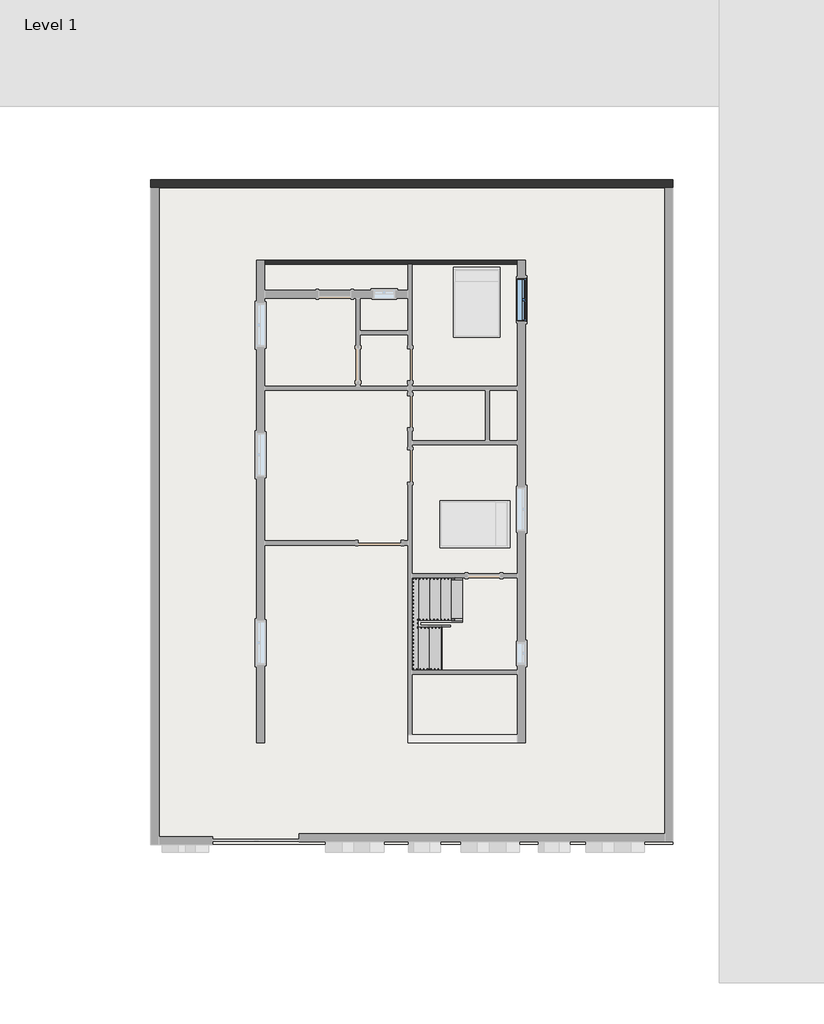
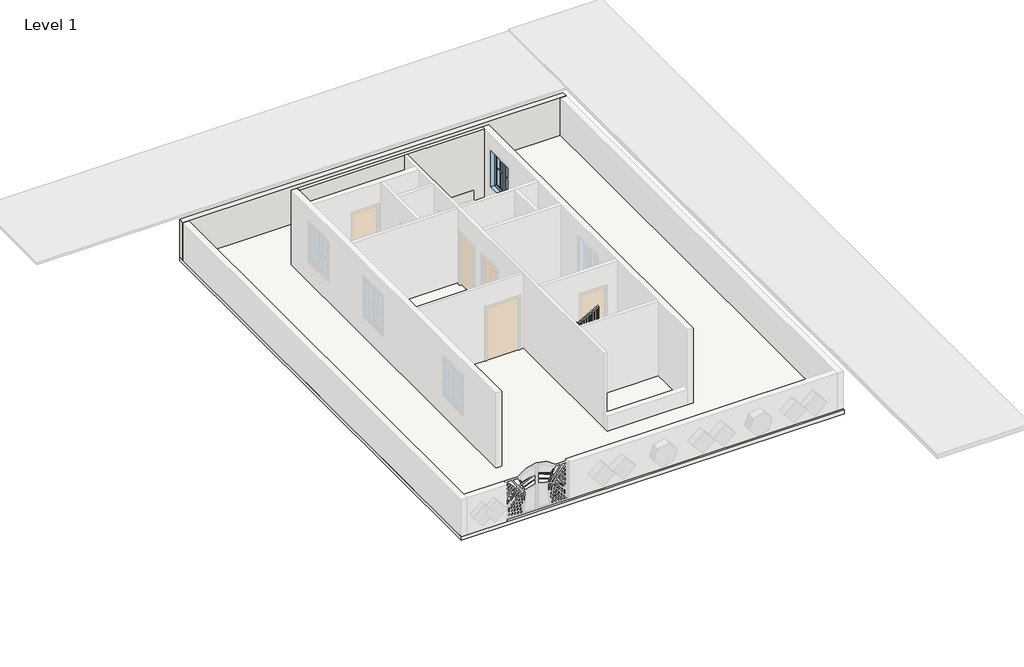
# One storey, part 2 of 7: 2 railings, 2 walls, 1 slab, 1 stair flight, 1 window.
"""IFC4 building model written with IfcOpenShell, lengths in millimetres."""

from ifc_helpers import new_model, si_unit, frame, origin, place, context, project, spatial, polyline, outline, extrude, faceted_brep, transform, mapped, element, save
from components import stair_flight_e4a46180, window_8377141f

model = new_model("IFC4")

# Units and contexts
model_context = context("Model", 3, world=origin())
ifc_project = project(units=[si_unit("LENGTHUNIT", "METRE", prefix="MILLI")], contexts=[model_context])

# Site, building, storey
site = spatial("IfcSite", under=ifc_project)
building = spatial("IfcBuilding", under=site)
storey = spatial("IfcBuildingStorey", under=building, Name="Level 1", Elevation=0.0)

# Railings
placement = place(None, origin())
element("IfcRailing", 1, ObjectType="Handrail - Rectangular", at=placement, inside=storey, context=model_context, shape_type="SolidModel", body=[
    faceted_brep([(7105.1820958, 5435.6, 1083.7333333), (7105.1820958, 5435.6, 1025.8977421), (7105.1820958, 5486.4, 1025.8977421), (7105.1820958, 5486.4, 1083.7333333), (5860.5820958, 5435.6, 1761.0666667), (5847.654197, 5435.6, 1710.2666667), (5847.654197, 5486.4, 1710.2666667), (5860.5820958, 5486.4, 1761.0666667), (5727.7, 5435.6, 1761.0666667), (5727.7, 5435.6, 1710.2666667), (5676.9, 5486.4, 1710.2666667), (5676.9, 5486.4, 1761.0666667), (5727.7, 2997.2, 1761.0666667), (5727.7, 2946.4, 1710.2666667), (5676.9, 2946.4, 1710.2666667), (5676.9, 2997.2, 1761.0666667), (5727.7, 2997.2, 1899.5526009), (5727.7, 2946.4, 1848.7526009), (5676.9, 2946.4, 1848.7526009), (5676.9, 2997.2, 1899.5526009), (5727.7, 2921.0, 1899.5526009), (5727.7, 2921.0, 1848.7526009), (5676.9, 2870.2, 1848.7526009), (5676.9, 2870.2, 1899.5526009), (5803.9, 2921.0, 1899.5526009), (5816.8278988, 2921.0, 1848.7526009), (5816.8278988, 2870.2, 1848.7526009), (5803.9, 2870.2, 1899.5526009), (7105.1820958, 2921.0, 2607.7333333), (7105.1820958, 2870.2, 2607.7333333), (7105.1820958, 2870.2, 2549.8977421), (7105.1820958, 2921.0, 2549.8977421)], [[[0, 1, 2, 3]], [[1, 0, 4, 5]], [[2, 1, 5, 6]], [[3, 2, 6, 7]], [[0, 3, 7, 4]], [[5, 4, 8, 9]], [[6, 5, 9, 10]], [[7, 6, 10, 11]], [[4, 7, 11, 8]], [[9, 8, 12, 13]], [[10, 9, 13, 14]], [[11, 10, 14, 15]], [[8, 11, 15, 12]], [[13, 12, 16, 17]], [[14, 13, 17, 18]], [[15, 14, 18, 19]], [[12, 15, 19, 16]], [[17, 16, 20, 21]], [[18, 17, 21, 22]], [[19, 18, 22, 23]], [[16, 19, 23, 20]], [[21, 20, 24, 25]], [[22, 21, 25, 26]], [[23, 22, 26, 27]], [[20, 23, 27, 24]], [[28, 29, 30, 31]], [[25, 24, 28, 31]], [[26, 25, 31, 30]], [[27, 26, 30, 29]], [[24, 27, 29, 28]]]),
    extrude(outline(polyline([(2510.4108873, 7032.625), (2500.0435403, 7013.575), (1524.0, 7013.575), (1524.0, 7032.625), (2510.4108873, 7032.625)])), frame((0.0, 2886.075, 0.0), z_axis=(0.0, 1.0, 0.0), x_axis=(0.0, 0.0, 1.0)), (0.0, 0.0, 1.0), 19.05),
    extrude(outline(polyline([(2455.1183703, 6931.025), (2444.7510233, 6911.975), (1524.0, 6911.975), (1524.0, 6931.025), (2455.1183703, 6931.025)])), frame((0.0, 2886.075, 0.0), z_axis=(0.0, 1.0, 0.0), x_axis=(0.0, 0.0, 1.0)), (0.0, 0.0, 1.0), 19.05),
    extrude(outline(polyline([(2399.8258533, 6829.425), (2389.4585063, 6810.375), (1524.0, 6810.375), (1524.0, 6829.425), (2399.8258533, 6829.425)])), frame((0.0, 2886.075, 0.0), z_axis=(0.0, 1.0, 0.0), x_axis=(0.0, 0.0, 1.0)), (0.0, 0.0, 1.0), 19.05),
    extrude(outline(polyline([(2344.5333363, 6727.825), (2334.1659893, 6708.775), (1354.6666667, 6708.775), (1354.6666667, 6727.825), (2344.5333363, 6727.825)])), frame((0.0, 2886.075, 0.0), z_axis=(0.0, 1.0, 0.0), x_axis=(0.0, 0.0, 1.0)), (0.0, 0.0, 1.0), 19.05),
    extrude(outline(polyline([(2289.2408192, 6626.225), (2278.8734723, 6607.175), (1354.6666667, 6607.175), (1354.6666667, 6626.225), (2289.2408192, 6626.225)])), frame((0.0, 2886.075, 0.0), z_axis=(0.0, 1.0, 0.0), x_axis=(0.0, 0.0, 1.0)), (0.0, 0.0, 1.0), 19.05),
    extrude(outline(polyline([(2233.9483022, 6524.625), (2223.5809553, 6505.575), (1354.6666667, 6505.575), (1354.6666667, 6524.625), (2233.9483022, 6524.625)])), frame((0.0, 2886.075, 0.0), z_axis=(0.0, 1.0, 0.0), x_axis=(0.0, 0.0, 1.0)), (0.0, 0.0, 1.0), 19.05),
    extrude(outline(polyline([(2178.6557852, 6423.025), (2168.2884383, 6403.975), (1185.3333333, 6403.975), (1185.3333333, 6423.025), (2178.6557852, 6423.025)])), frame((0.0, 2886.075, 0.0), z_axis=(0.0, 1.0, 0.0), x_axis=(0.0, 0.0, 1.0)), (0.0, 0.0, 1.0), 19.05),
    extrude(outline(polyline([(2123.3632682, 6321.425), (2112.9959213, 6302.375), (1185.3333333, 6302.375), (1185.3333333, 6321.425), (2123.3632682, 6321.425)])), frame((0.0, 2886.075, 0.0), z_axis=(0.0, 1.0, 0.0), x_axis=(0.0, 0.0, 1.0)), (0.0, 0.0, 1.0), 19.05),
    extrude(outline(polyline([(2068.0707512, 6219.825), (2057.7034043, 6200.775), (1185.3333333, 6200.775), (1185.3333333, 6219.825), (2068.0707512, 6219.825)])), frame((0.0, 2886.075, 0.0), z_axis=(0.0, 1.0, 0.0), x_axis=(0.0, 0.0, 1.0)), (0.0, 0.0, 1.0), 19.05),
    extrude(outline(polyline([(2012.7782342, 6118.225), (2002.4108873, 6099.175), (1016.0, 6099.175), (1016.0, 6118.225), (2012.7782342, 6118.225)])), frame((0.0, 2886.075, 0.0), z_axis=(0.0, 1.0, 0.0), x_axis=(0.0, 0.0, 1.0)), (0.0, 0.0, 1.0), 19.05),
    extrude(outline(polyline([(1957.4857172, 6016.625), (1947.1183703, 5997.575), (1016.0, 5997.575), (1016.0, 6016.625), (1957.4857172, 6016.625)])), frame((0.0, 2886.075, 0.0), z_axis=(0.0, 1.0, 0.0), x_axis=(0.0, 0.0, 1.0)), (0.0, 0.0, 1.0), 19.05),
    extrude(outline(polyline([(1902.1932002, 5915.025), (1891.8258533, 5895.975), (1016.0, 5895.975), (1016.0, 5915.025), (1902.1932002, 5915.025)])), frame((0.0, 2886.075, 0.0), z_axis=(0.0, 1.0, 0.0), x_axis=(0.0, 0.0, 1.0)), (0.0, 0.0, 1.0), 19.05),
    extrude(outline(polyline([(1846.9006832, 5813.425), (1836.5333363, 5794.375), (846.6666667, 5794.375), (846.6666667, 5813.425), (1846.9006832, 5813.425)])), frame((0.0, 2886.075, 0.0), z_axis=(0.0, 1.0, 0.0), x_axis=(0.0, 0.0, 1.0)), (0.0, 0.0, 1.0), 19.05),
    extrude(outline(polyline([(5692.775, 2930.525), (5711.825, 2930.525), (5711.825, 2911.475), (5692.775, 2911.475), (5692.775, 2930.525)])), frame((0.0, 0.0, 846.6666667), z_axis=(0.0, 0.0, 1.0), x_axis=(1.0, 0.0, 0.0)), (0.0, 0.0, 1.0), 1002.0859343),
    extrude(outline(polyline([(5692.775, 3032.125), (5711.825, 3032.125), (5711.825, 3013.075), (5692.775, 3013.075), (5692.775, 3032.125)])), frame((0.0, 0.0, 846.6666667), z_axis=(0.0, 0.0, 1.0), x_axis=(1.0, 0.0, 0.0)), (0.0, 0.0, 1.0), 863.6),
    extrude(outline(polyline([(5692.775, 3133.725), (5711.825, 3133.725), (5711.825, 3114.675), (5692.775, 3114.675), (5692.775, 3133.725)])), frame((0.0, 0.0, 846.6666667), z_axis=(0.0, 0.0, 1.0), x_axis=(1.0, 0.0, 0.0)), (0.0, 0.0, 1.0), 863.6),
    extrude(outline(polyline([(5692.775, 3235.325), (5711.825, 3235.325), (5711.825, 3216.275), (5692.775, 3216.275), (5692.775, 3235.325)])), frame((0.0, 0.0, 846.6666667), z_axis=(0.0, 0.0, 1.0), x_axis=(1.0, 0.0, 0.0)), (0.0, 0.0, 1.0), 863.6),
    extrude(outline(polyline([(5692.775, 3336.925), (5711.825, 3336.925), (5711.825, 3317.875), (5692.775, 3317.875), (5692.775, 3336.925)])), frame((0.0, 0.0, 846.6666667), z_axis=(0.0, 0.0, 1.0), x_axis=(1.0, 0.0, 0.0)), (0.0, 0.0, 1.0), 863.6),
    extrude(outline(polyline([(5692.775, 3438.525), (5711.825, 3438.525), (5711.825, 3419.475), (5692.775, 3419.475), (5692.775, 3438.525)])), frame((0.0, 0.0, 846.6666667), z_axis=(0.0, 0.0, 1.0), x_axis=(1.0, 0.0, 0.0)), (0.0, 0.0, 1.0), 863.6),
    extrude(outline(polyline([(5692.775, 3540.125), (5711.825, 3540.125), (5711.825, 3521.075), (5692.775, 3521.075), (5692.775, 3540.125)])), frame((0.0, 0.0, 846.6666667), z_axis=(0.0, 0.0, 1.0), x_axis=(1.0, 0.0, 0.0)), (0.0, 0.0, 1.0), 863.6),
    extrude(outline(polyline([(5692.775, 3641.725), (5711.825, 3641.725), (5711.825, 3622.675), (5692.775, 3622.675), (5692.775, 3641.725)])), frame((0.0, 0.0, 846.6666667), z_axis=(0.0, 0.0, 1.0), x_axis=(1.0, 0.0, 0.0)), (0.0, 0.0, 1.0), 863.6),
    extrude(outline(polyline([(5692.775, 3743.325), (5711.825, 3743.325), (5711.825, 3724.275), (5692.775, 3724.275), (5692.775, 3743.325)])), frame((0.0, 0.0, 846.6666667), z_axis=(0.0, 0.0, 1.0), x_axis=(1.0, 0.0, 0.0)), (0.0, 0.0, 1.0), 863.6),
    extrude(outline(polyline([(5692.775, 3844.925), (5711.825, 3844.925), (5711.825, 3825.875), (5692.775, 3825.875), (5692.775, 3844.925)])), frame((0.0, 0.0, 846.6666667), z_axis=(0.0, 0.0, 1.0), x_axis=(1.0, 0.0, 0.0)), (0.0, 0.0, 1.0), 863.6),
    extrude(outline(polyline([(5692.775, 3946.525), (5711.825, 3946.525), (5711.825, 3927.475), (5692.775, 3927.475), (5692.775, 3946.525)])), frame((0.0, 0.0, 846.6666667), z_axis=(0.0, 0.0, 1.0), x_axis=(1.0, 0.0, 0.0)), (0.0, 0.0, 1.0), 863.6),
    extrude(outline(polyline([(5692.775, 4048.125), (5711.825, 4048.125), (5711.825, 4029.075), (5692.775, 4029.075), (5692.775, 4048.125)])), frame((0.0, 0.0, 846.6666667), z_axis=(0.0, 0.0, 1.0), x_axis=(1.0, 0.0, 0.0)), (0.0, 0.0, 1.0), 863.6),
    extrude(outline(polyline([(5692.775, 4149.725), (5711.825, 4149.725), (5711.825, 4130.675), (5692.775, 4130.675), (5692.775, 4149.725)])), frame((0.0, 0.0, 846.6666667), z_axis=(0.0, 0.0, 1.0), x_axis=(1.0, 0.0, 0.0)), (0.0, 0.0, 1.0), 863.6),
    extrude(outline(polyline([(5692.775, 4251.325), (5711.825, 4251.325), (5711.825, 4232.275), (5692.775, 4232.275), (5692.775, 4251.325)])), frame((0.0, 0.0, 846.6666667), z_axis=(0.0, 0.0, 1.0), x_axis=(1.0, 0.0, 0.0)), (0.0, 0.0, 1.0), 863.6),
    extrude(outline(polyline([(5692.775, 4352.925), (5711.825, 4352.925), (5711.825, 4333.875), (5692.775, 4333.875), (5692.775, 4352.925)])), frame((0.0, 0.0, 846.6666667), z_axis=(0.0, 0.0, 1.0), x_axis=(1.0, 0.0, 0.0)), (0.0, 0.0, 1.0), 863.6),
    extrude(outline(polyline([(5692.775, 4454.525), (5711.825, 4454.525), (5711.825, 4435.475), (5692.775, 4435.475), (5692.775, 4454.525)])), frame((0.0, 0.0, 846.6666667), z_axis=(0.0, 0.0, 1.0), x_axis=(1.0, 0.0, 0.0)), (0.0, 0.0, 1.0), 863.6),
    extrude(outline(polyline([(5692.775, 4556.125), (5711.825, 4556.125), (5711.825, 4537.075), (5692.775, 4537.075), (5692.775, 4556.125)])), frame((0.0, 0.0, 846.6666667), z_axis=(0.0, 0.0, 1.0), x_axis=(1.0, 0.0, 0.0)), (0.0, 0.0, 1.0), 863.6),
    extrude(outline(polyline([(5692.775, 4657.725), (5711.825, 4657.725), (5711.825, 4638.675), (5692.775, 4638.675), (5692.775, 4657.725)])), frame((0.0, 0.0, 846.6666667), z_axis=(0.0, 0.0, 1.0), x_axis=(1.0, 0.0, 0.0)), (0.0, 0.0, 1.0), 863.6),
    extrude(outline(polyline([(5692.775, 4759.325), (5711.825, 4759.325), (5711.825, 4740.275), (5692.775, 4740.275), (5692.775, 4759.325)])), frame((0.0, 0.0, 846.6666667), z_axis=(0.0, 0.0, 1.0), x_axis=(1.0, 0.0, 0.0)), (0.0, 0.0, 1.0), 863.6),
    extrude(outline(polyline([(5692.775, 4860.925), (5711.825, 4860.925), (5711.825, 4841.875), (5692.775, 4841.875), (5692.775, 4860.925)])), frame((0.0, 0.0, 846.6666667), z_axis=(0.0, 0.0, 1.0), x_axis=(1.0, 0.0, 0.0)), (0.0, 0.0, 1.0), 863.6),
    extrude(outline(polyline([(5692.775, 4962.525), (5711.825, 4962.525), (5711.825, 4943.475), (5692.775, 4943.475), (5692.775, 4962.525)])), frame((0.0, 0.0, 846.6666667), z_axis=(0.0, 0.0, 1.0), x_axis=(1.0, 0.0, 0.0)), (0.0, 0.0, 1.0), 863.6),
    extrude(outline(polyline([(5692.775, 5064.125), (5711.825, 5064.125), (5711.825, 5045.075), (5692.775, 5045.075), (5692.775, 5064.125)])), frame((0.0, 0.0, 846.6666667), z_axis=(0.0, 0.0, 1.0), x_axis=(1.0, 0.0, 0.0)), (0.0, 0.0, 1.0), 863.6),
    extrude(outline(polyline([(5692.775, 5165.725), (5711.825, 5165.725), (5711.825, 5146.675), (5692.775, 5146.675), (5692.775, 5165.725)])), frame((0.0, 0.0, 846.6666667), z_axis=(0.0, 0.0, 1.0), x_axis=(1.0, 0.0, 0.0)), (0.0, 0.0, 1.0), 863.6),
    extrude(outline(polyline([(5692.775, 5267.325), (5711.825, 5267.325), (5711.825, 5248.275), (5692.775, 5248.275), (5692.775, 5267.325)])), frame((0.0, 0.0, 846.6666667), z_axis=(0.0, 0.0, 1.0), x_axis=(1.0, 0.0, 0.0)), (0.0, 0.0, 1.0), 863.6),
    extrude(outline(polyline([(5692.775, 5368.925), (5711.825, 5368.925), (5711.825, 5349.875), (5692.775, 5349.875), (5692.775, 5368.925)])), frame((0.0, 0.0, 846.6666667), z_axis=(0.0, 0.0, 1.0), x_axis=(1.0, 0.0, 0.0)), (0.0, 0.0, 1.0), 863.6),
    extrude(outline(polyline([(5793.9070958, 5470.525), (5793.9070958, 5451.475), (5774.8570958, 5451.475), (5774.8570958, 5470.525), (5793.9070958, 5470.525)])), frame((0.0, 0.0, 846.6666667), z_axis=(0.0, 0.0, 1.0), x_axis=(1.0, 0.0, 0.0)), (0.0, 0.0, 1.0), 863.6),
    extrude(outline(polyline([(1684.2242727, 5895.5070958), (1694.5916197, 5876.4570958), (677.3333333, 5876.4570958), (677.3333333, 5895.5070958), (1684.2242727, 5895.5070958)])), frame((0.0, 5451.475, 0.0), z_axis=(0.0, 1.0, 0.0), x_axis=(0.0, 0.0, 1.0)), (0.0, 0.0, 1.0), 19.05),
    extrude(outline(polyline([(1628.9317557, 5997.1070958), (1639.2991027, 5978.0570958), (677.3333333, 5978.0570958), (677.3333333, 5997.1070958), (1628.9317557, 5997.1070958)])), frame((0.0, 5451.475, 0.0), z_axis=(0.0, 1.0, 0.0), x_axis=(0.0, 0.0, 1.0)), (0.0, 0.0, 1.0), 19.05),
    extrude(outline(polyline([(1573.6392387, 6098.7070958), (1584.0065857, 6079.6570958), (677.3333333, 6079.6570958), (677.3333333, 6098.7070958), (1573.6392387, 6098.7070958)])), frame((0.0, 5451.475, 0.0), z_axis=(0.0, 1.0, 0.0), x_axis=(0.0, 0.0, 1.0)), (0.0, 0.0, 1.0), 19.05),
    extrude(outline(polyline([(1518.3467217, 6200.3070958), (1528.7140687, 6181.2570958), (508.0, 6181.2570958), (508.0, 6200.3070958), (1518.3467217, 6200.3070958)])), frame((0.0, 5451.475, 0.0), z_axis=(0.0, 1.0, 0.0), x_axis=(0.0, 0.0, 1.0)), (0.0, 0.0, 1.0), 19.05),
    extrude(outline(polyline([(1463.0542047, 6301.9070958), (1473.4215517, 6282.8570958), (508.0, 6282.8570958), (508.0, 6301.9070958), (1463.0542047, 6301.9070958)])), frame((0.0, 5451.475, 0.0), z_axis=(0.0, 1.0, 0.0), x_axis=(0.0, 0.0, 1.0)), (0.0, 0.0, 1.0), 19.05),
    extrude(outline(polyline([(1407.7616877, 6403.5070958), (1418.1290347, 6384.4570958), (508.0, 6384.4570958), (508.0, 6403.5070958), (1407.7616877, 6403.5070958)])), frame((0.0, 5451.475, 0.0), z_axis=(0.0, 1.0, 0.0), x_axis=(0.0, 0.0, 1.0)), (0.0, 0.0, 1.0), 19.05),
    extrude(outline(polyline([(1352.4691707, 6505.1070958), (1362.8365176, 6486.0570958), (338.6666667, 6486.0570958), (338.6666667, 6505.1070958), (1352.4691707, 6505.1070958)])), frame((0.0, 5451.475, 0.0), z_axis=(0.0, 1.0, 0.0), x_axis=(0.0, 0.0, 1.0)), (0.0, 0.0, 1.0), 19.05),
    extrude(outline(polyline([(1297.1766537, 6606.7070958), (1307.5440006, 6587.6570958), (338.6666667, 6587.6570958), (338.6666667, 6606.7070958), (1297.1766537, 6606.7070958)])), frame((0.0, 5451.475, 0.0), z_axis=(0.0, 1.0, 0.0), x_axis=(0.0, 0.0, 1.0)), (0.0, 0.0, 1.0), 19.05),
    extrude(outline(polyline([(1241.8841367, 6708.3070958), (1252.2514836, 6689.2570958), (338.6666667, 6689.2570958), (338.6666667, 6708.3070958), (1241.8841367, 6708.3070958)])), frame((0.0, 5451.475, 0.0), z_axis=(0.0, 1.0, 0.0), x_axis=(0.0, 0.0, 1.0)), (0.0, 0.0, 1.0), 19.05),
    extrude(outline(polyline([(1186.5916197, 6809.9070958), (1196.9589666, 6790.8570958), (169.3333333, 6790.8570958), (169.3333333, 6809.9070958), (1186.5916197, 6809.9070958)])), frame((0.0, 5451.475, 0.0), z_axis=(0.0, 1.0, 0.0), x_axis=(0.0, 0.0, 1.0)), (0.0, 0.0, 1.0), 19.05),
    extrude(outline(polyline([(1131.2991027, 6911.5070958), (1141.6664496, 6892.4570958), (169.3333333, 6892.4570958), (169.3333333, 6911.5070958), (1131.2991027, 6911.5070958)])), frame((0.0, 5451.475, 0.0), z_axis=(0.0, 1.0, 0.0), x_axis=(0.0, 0.0, 1.0)), (0.0, 0.0, 1.0), 19.05),
    extrude(outline(polyline([(1076.0065857, 7013.1070958), (1086.3739326, 6994.0570958), (169.3333333, 6994.0570958), (169.3333333, 7013.1070958), (1076.0065857, 7013.1070958)])), frame((0.0, 5451.475, 0.0), z_axis=(0.0, 1.0, 0.0), x_axis=(0.0, 0.0, 1.0)), (0.0, 0.0, 1.0), 19.05),
    extrude(outline(polyline([(5692.775, 2905.125), (5711.825, 2905.125), (5711.825, 2886.075), (5692.775, 2886.075), (5692.775, 2905.125)])), frame((0.0, 0.0, 846.6666667), z_axis=(0.0, 0.0, 1.0), x_axis=(1.0, 0.0, 0.0)), (0.0, 0.0, 1.0), 1002.0859343),
    extrude(outline(polyline([(5711.825, 5470.525), (5711.825, 5451.475), (5692.775, 5451.475), (5692.775, 5470.525), (5711.825, 5470.525)])), frame((0.0, 0.0, 846.6666667), z_axis=(0.0, 0.0, 1.0), x_axis=(1.0, 0.0, 0.0)), (0.0, 0.0, 1.0), 863.6),
    extrude(outline(polyline([(2549.8977421, 7105.1820958), (2539.5303952, 7086.1320958), (1524.0, 7086.1320958), (1524.0, 7105.1820958), (2549.8977421, 7105.1820958)])), frame((0.0, 2886.075, 0.0), z_axis=(0.0, 1.0, 0.0), x_axis=(0.0, 0.0, 1.0)), (0.0, 0.0, 1.0), 19.05),
    extrude(outline(polyline([(1025.8977421, 7105.1820958), (1036.2650891, 7086.1320958), (169.3333333, 7086.1320958), (169.3333333, 7105.1820958), (1025.8977421, 7105.1820958)])), frame((0.0, 5451.475, 0.0), z_axis=(0.0, 1.0, 0.0), x_axis=(0.0, 0.0, 1.0)), (0.0, 0.0, 1.0), 19.05),
])
element("IfcRailing", 2, ObjectType="Handrail - Rectangular", at=placement, inside=storey, context=model_context, shape_type="SolidModel", body=[
    faceted_brep([(7105.1820958, 4274.6882626, 1083.7333333), (7105.1820958, 4274.6882626, 1025.8977421), (7105.1820958, 4325.4882626, 1025.8977421), (7105.1820958, 4325.4882626, 1083.7333333), (5936.7820958, 4274.6882626, 1719.5972789), (5885.9820958, 4274.6882626, 1689.4079462), (5885.9820958, 4325.4882626, 1689.4079462), (5936.7820958, 4325.4882626, 1719.5972789), (5936.7820958, 4274.6882626, 1761.0666667), (5885.9820958, 4274.6882626, 1710.2666667), (5885.9820958, 4325.4882626, 1710.2666667), (5936.7820958, 4325.4882626, 1761.0666667), (5860.5820958, 4274.6882626, 1761.0666667), (5860.5820958, 4274.6882626, 1710.2666667), (5809.7820958, 4325.4882626, 1710.2666667), (5809.7820958, 4325.4882626, 1761.0666667), (5860.5820958, 4198.4882626, 1761.0666667), (5860.5820958, 4198.4882626, 1710.2666667), (5809.7820958, 4198.4882626, 1710.2666667), (5809.7820958, 4198.4882626, 1761.0666667), (5860.5820958, 4173.0882626, 1761.0666667), (5860.5820958, 4122.2882626, 1710.2666667), (5809.7820958, 4122.2882626, 1710.2666667), (5809.7820958, 4173.0882626, 1761.0666667), (5860.5820958, 4173.0882626, 1971.8693878), (5860.5820958, 4122.2882626, 1921.0693878), (5809.7820958, 4122.2882626, 1921.0693878), (5809.7820958, 4173.0882626, 1971.8693878), (5860.5820958, 4096.8882626, 1971.8693878), (5860.5820958, 4096.8882626, 1921.0693878), (5809.7820958, 4046.0882626, 1921.0693878), (5809.7820958, 4046.0882626, 1971.8693878), (5936.7820958, 4096.8882626, 1971.8693878), (5949.7099946, 4096.8882626, 1921.0693878), (5949.7099946, 4046.0882626, 1921.0693878), (5936.7820958, 4046.0882626, 1971.8693878), (7105.1820958, 4096.8882626, 2607.7333333), (7105.1820958, 4046.0882626, 2607.7333333), (7105.1820958, 4046.0882626, 2549.8977421), (7105.1820958, 4096.8882626, 2549.8977421)], [[[0, 1, 2, 3]], [[1, 0, 4, 5]], [[2, 1, 5, 6]], [[3, 2, 6, 7]], [[0, 3, 7, 4]], [[5, 4, 8, 9]], [[6, 5, 9, 10]], [[7, 6, 10, 11]], [[4, 7, 11, 8]], [[9, 8, 12, 13]], [[10, 9, 13, 14]], [[11, 10, 14, 15]], [[8, 11, 15, 12]], [[13, 12, 16, 17]], [[14, 13, 17, 18]], [[15, 14, 18, 19]], [[12, 15, 19, 16]], [[17, 16, 20, 21]], [[18, 17, 21, 22]], [[19, 18, 22, 23]], [[16, 19, 23, 20]], [[21, 20, 24, 25]], [[22, 21, 25, 26]], [[23, 22, 26, 27]], [[20, 23, 27, 24]], [[25, 24, 28, 29]], [[26, 25, 29, 30]], [[27, 26, 30, 31]], [[24, 27, 31, 28]], [[29, 28, 32, 33]], [[30, 29, 33, 34]], [[31, 30, 34, 35]], [[28, 31, 35, 32]], [[36, 37, 38, 39]], [[33, 32, 36, 39]], [[34, 33, 39, 38]], [[35, 34, 38, 37]], [[32, 35, 37, 36]]]),
    extrude(outline(polyline([(2517.0678102, 7044.8570958), (1524.0, 7044.8570958), (1524.0, 7063.9070958), (2527.4351571, 7063.9070958), (2517.0678102, 7044.8570958)])), frame((0.0, 4061.9632626, 0.0), z_axis=(0.0, 1.0, 0.0), x_axis=(0.0, 0.0, 1.0)), (0.0, 0.0, 1.0), 19.05),
    extrude(outline(polyline([(2461.7752932, 6943.2570958), (1524.0, 6943.2570958), (1524.0, 6962.3070958), (2472.1426401, 6962.3070958), (2461.7752932, 6943.2570958)])), frame((0.0, 4061.9632626, 0.0), z_axis=(0.0, 1.0, 0.0), x_axis=(0.0, 0.0, 1.0)), (0.0, 0.0, 1.0), 19.05),
    extrude(outline(polyline([(2406.4827761, 6841.6570958), (1524.0, 6841.6570958), (1524.0, 6860.7070958), (2416.8501231, 6860.7070958), (2406.4827761, 6841.6570958)])), frame((0.0, 4061.9632626, 0.0), z_axis=(0.0, 1.0, 0.0), x_axis=(0.0, 0.0, 1.0)), (0.0, 0.0, 1.0), 19.05),
    extrude(outline(polyline([(2351.1902591, 6740.0570958), (1354.6666667, 6740.0570958), (1354.6666667, 6759.1070958), (2361.5576061, 6759.1070958), (2351.1902591, 6740.0570958)])), frame((0.0, 4061.9632626, 0.0), z_axis=(0.0, 1.0, 0.0), x_axis=(0.0, 0.0, 1.0)), (0.0, 0.0, 1.0), 19.05),
    extrude(outline(polyline([(2295.8977421, 6638.4570958), (1354.6666667, 6638.4570958), (1354.6666667, 6657.5070958), (2306.2650891, 6657.5070958), (2295.8977421, 6638.4570958)])), frame((0.0, 4061.9632626, 0.0), z_axis=(0.0, 1.0, 0.0), x_axis=(0.0, 0.0, 1.0)), (0.0, 0.0, 1.0), 19.05),
    extrude(outline(polyline([(2240.6052251, 6536.8570958), (1354.6666667, 6536.8570958), (1354.6666667, 6555.9070958), (2250.9725721, 6555.9070958), (2240.6052251, 6536.8570958)])), frame((0.0, 4061.9632626, 0.0), z_axis=(0.0, 1.0, 0.0), x_axis=(0.0, 0.0, 1.0)), (0.0, 0.0, 1.0), 19.05),
    extrude(outline(polyline([(2185.3127081, 6435.2570958), (1185.3333333, 6435.2570958), (1185.3333333, 6454.3070958), (2195.6800551, 6454.3070958), (2185.3127081, 6435.2570958)])), frame((0.0, 4061.9632626, 0.0), z_axis=(0.0, 1.0, 0.0), x_axis=(0.0, 0.0, 1.0)), (0.0, 0.0, 1.0), 19.05),
    extrude(outline(polyline([(2130.0201911, 6333.6570958), (1185.3333333, 6333.6570958), (1185.3333333, 6352.7070958), (2140.3875381, 6352.7070958), (2130.0201911, 6333.6570958)])), frame((0.0, 4061.9632626, 0.0), z_axis=(0.0, 1.0, 0.0), x_axis=(0.0, 0.0, 1.0)), (0.0, 0.0, 1.0), 19.05),
    extrude(outline(polyline([(2074.7276741, 6232.0570958), (1185.3333333, 6232.0570958), (1185.3333333, 6251.1070958), (2085.095021, 6251.1070958), (2074.7276741, 6232.0570958)])), frame((0.0, 4061.9632626, 0.0), z_axis=(0.0, 1.0, 0.0), x_axis=(0.0, 0.0, 1.0)), (0.0, 0.0, 1.0), 19.05),
    extrude(outline(polyline([(2019.4351571, 6130.4570958), (1016.0, 6130.4570958), (1016.0, 6149.5070958), (2029.802504, 6149.5070958), (2019.4351571, 6130.4570958)])), frame((0.0, 4061.9632626, 0.0), z_axis=(0.0, 1.0, 0.0), x_axis=(0.0, 0.0, 1.0)), (0.0, 0.0, 1.0), 19.05),
    extrude(outline(polyline([(1964.1426401, 6028.8570958), (1016.0, 6028.8570958), (1016.0, 6047.9070958), (1974.509987, 6047.9070958), (1964.1426401, 6028.8570958)])), frame((0.0, 4061.9632626, 0.0), z_axis=(0.0, 1.0, 0.0), x_axis=(0.0, 0.0, 1.0)), (0.0, 0.0, 1.0), 19.05),
    extrude(outline(polyline([(1908.8501231, 5927.2570958), (1016.0, 5927.2570958), (1016.0, 5946.3070958), (1919.21747, 5946.3070958), (1908.8501231, 5927.2570958)])), frame((0.0, 4061.9632626, 0.0), z_axis=(0.0, 1.0, 0.0), x_axis=(0.0, 0.0, 1.0)), (0.0, 0.0, 1.0), 19.05),
    extrude(outline(polyline([(5844.7070958, 4106.4132626), (5844.7070958, 4087.3632626), (5825.6570958, 4087.3632626), (5825.6570958, 4106.4132626), (5844.7070958, 4106.4132626)])), frame((0.0, 0.0, 846.6666667), z_axis=(0.0, 0.0, 1.0), x_axis=(1.0, 0.0, 0.0)), (0.0, 0.0, 1.0), 1074.4027211),
    extrude(outline(polyline([(5844.7070958, 4208.0132626), (5844.7070958, 4188.9632626), (5825.6570958, 4188.9632626), (5825.6570958, 4208.0132626), (5844.7070958, 4208.0132626)])), frame((0.0, 0.0, 846.6666667), z_axis=(0.0, 0.0, 1.0), x_axis=(1.0, 0.0, 0.0)), (0.0, 0.0, 1.0), 863.6),
    extrude(outline(polyline([(5895.5070958, 4290.5632626), (5876.4570958, 4290.5632626), (5876.4570958, 4309.6132626), (5895.5070958, 4309.6132626), (5895.5070958, 4290.5632626)])), frame((0.0, 0.0, 677.3333333), z_axis=(0.0, 0.0, 1.0), x_axis=(1.0, 0.0, 0.0)), (0.0, 0.0, 1.0), 1032.9333333),
    extrude(outline(polyline([(1639.2991027, 5978.0570958), (677.3333333, 5978.0570958), (677.3333333, 5997.1070958), (1628.9317557, 5997.1070958), (1639.2991027, 5978.0570958)])), frame((0.0, 4290.5632626, 0.0), z_axis=(0.0, 1.0, 0.0), x_axis=(0.0, 0.0, 1.0)), (0.0, 0.0, 1.0), 19.05),
    extrude(outline(polyline([(1584.0065857, 6079.6570958), (677.3333333, 6079.6570958), (677.3333333, 6098.7070958), (1573.6392387, 6098.7070958), (1584.0065857, 6079.6570958)])), frame((0.0, 4290.5632626, 0.0), z_axis=(0.0, 1.0, 0.0), x_axis=(0.0, 0.0, 1.0)), (0.0, 0.0, 1.0), 19.05),
    extrude(outline(polyline([(1528.7140687, 6181.2570958), (508.0, 6181.2570958), (508.0, 6200.3070958), (1518.3467217, 6200.3070958), (1528.7140687, 6181.2570958)])), frame((0.0, 4290.5632626, 0.0), z_axis=(0.0, 1.0, 0.0), x_axis=(0.0, 0.0, 1.0)), (0.0, 0.0, 1.0), 19.05),
    extrude(outline(polyline([(1473.4215517, 6282.8570958), (508.0, 6282.8570958), (508.0, 6301.9070958), (1463.0542047, 6301.9070958), (1473.4215517, 6282.8570958)])), frame((0.0, 4290.5632626, 0.0), z_axis=(0.0, 1.0, 0.0), x_axis=(0.0, 0.0, 1.0)), (0.0, 0.0, 1.0), 19.05),
    extrude(outline(polyline([(1418.1290347, 6384.4570958), (508.0, 6384.4570958), (508.0, 6403.5070958), (1407.7616877, 6403.5070958), (1418.1290347, 6384.4570958)])), frame((0.0, 4290.5632626, 0.0), z_axis=(0.0, 1.0, 0.0), x_axis=(0.0, 0.0, 1.0)), (0.0, 0.0, 1.0), 19.05),
    extrude(outline(polyline([(1362.8365176, 6486.0570958), (338.6666667, 6486.0570958), (338.6666667, 6505.1070958), (1352.4691707, 6505.1070958), (1362.8365176, 6486.0570958)])), frame((0.0, 4290.5632626, 0.0), z_axis=(0.0, 1.0, 0.0), x_axis=(0.0, 0.0, 1.0)), (0.0, 0.0, 1.0), 19.05),
    extrude(outline(polyline([(1307.5440006, 6587.6570958), (338.6666667, 6587.6570958), (338.6666667, 6606.7070958), (1297.1766537, 6606.7070958), (1307.5440006, 6587.6570958)])), frame((0.0, 4290.5632626, 0.0), z_axis=(0.0, 1.0, 0.0), x_axis=(0.0, 0.0, 1.0)), (0.0, 0.0, 1.0), 19.05),
    extrude(outline(polyline([(1252.2514836, 6689.2570958), (338.6666667, 6689.2570958), (338.6666667, 6708.3070958), (1241.8841367, 6708.3070958), (1252.2514836, 6689.2570958)])), frame((0.0, 4290.5632626, 0.0), z_axis=(0.0, 1.0, 0.0), x_axis=(0.0, 0.0, 1.0)), (0.0, 0.0, 1.0), 19.05),
    extrude(outline(polyline([(1196.9589666, 6790.8570958), (169.3333333, 6790.8570958), (169.3333333, 6809.9070958), (1186.5916197, 6809.9070958), (1196.9589666, 6790.8570958)])), frame((0.0, 4290.5632626, 0.0), z_axis=(0.0, 1.0, 0.0), x_axis=(0.0, 0.0, 1.0)), (0.0, 0.0, 1.0), 19.05),
    extrude(outline(polyline([(1141.6664496, 6892.4570958), (169.3333333, 6892.4570958), (169.3333333, 6911.5070958), (1131.2991027, 6911.5070958), (1141.6664496, 6892.4570958)])), frame((0.0, 4290.5632626, 0.0), z_axis=(0.0, 1.0, 0.0), x_axis=(0.0, 0.0, 1.0)), (0.0, 0.0, 1.0), 19.05),
    extrude(outline(polyline([(1086.3739326, 6994.0570958), (169.3333333, 6994.0570958), (169.3333333, 7013.1070958), (1076.0065857, 7013.1070958), (1086.3739326, 6994.0570958)])), frame((0.0, 4290.5632626, 0.0), z_axis=(0.0, 1.0, 0.0), x_axis=(0.0, 0.0, 1.0)), (0.0, 0.0, 1.0), 19.05),
    extrude(outline(polyline([(5844.7070958, 4081.0132626), (5844.7070958, 4061.9632626), (5825.6570958, 4061.9632626), (5825.6570958, 4081.0132626), (5844.7070958, 4081.0132626)])), frame((0.0, 0.0, 846.6666667), z_axis=(0.0, 0.0, 1.0), x_axis=(1.0, 0.0, 0.0)), (0.0, 0.0, 1.0), 1074.4027211),
    extrude(outline(polyline([(5844.7070958, 4290.5632626), (5825.6570958, 4290.5632626), (5825.6570958, 4309.6132626), (5844.7070958, 4309.6132626), (5844.7070958, 4290.5632626)])), frame((0.0, 0.0, 846.6666667), z_axis=(0.0, 0.0, 1.0), x_axis=(1.0, 0.0, 0.0)), (0.0, 0.0, 1.0), 863.6),
    extrude(outline(polyline([(2539.5303952, 7086.1320958), (1524.0, 7086.1320958), (1524.0, 7105.1820958), (2549.8977421, 7105.1820958), (2539.5303952, 7086.1320958)])), frame((0.0, 4061.9632626, 0.0), z_axis=(0.0, 1.0, 0.0), x_axis=(0.0, 0.0, 1.0)), (0.0, 0.0, 1.0), 19.05),
    extrude(outline(polyline([(1036.2650891, 7086.1320958), (169.3333333, 7086.1320958), (169.3333333, 7105.1820958), (1025.8977421, 7105.1820958), (1036.2650891, 7086.1320958)])), frame((0.0, 4290.5632626, 0.0), z_axis=(0.0, 1.0, 0.0), x_axis=(0.0, 0.0, 1.0)), (0.0, 0.0, 1.0), 19.05),
])

# Slab
element("IfcSlab", 3, ObjectType="Generic - 12\"", at=placement, inside=storey, context=model_context, shape_type="SweptSolid", body=[
    extrude(outline(polyline([(13056.5234142, 16761.595404), (13056.5234142, -2063.75), (-1726.2765858, -2063.75), (-1726.2765858, 16761.595404), (13056.5234142, 16761.595404)])), frame((0.0, 0.0, -152.4), z_axis=(0.0, 0.0, 1.0), x_axis=(1.0, 0.0, 0.0)), (0.0, 0.0, 1.0), 152.4),
])

# Stair flight
stair_flight_shape = stair_flight_e4a46180(model_context)
element("IfcStairFlight", 4, ObjectType="2\" Tread 1\" Nosing 1/4\" Riser", at=placement, inside=storey, context=model_context, shape_type="MappedRepresentation", body=[
    mapped(stair_flight_shape, transform((0.0, 0.0, 0.0), x_axis=(1.0, 0.0, 0.0), y_axis=(0.0, 1.0, 0.0), z_axis=(0.0, 0.0, 1.0))),
])

# Walls
element("IfcWall", 5, ObjectType="Generic - 5\"", at=placement, inside=storey, context=model_context, shape_type="Brep", body=[
    faceted_brep([(1498.6, 14363.7, 0.0), (5562.6, 14363.7, 0.0), (5676.9, 14363.7, 0.0), (8661.4, 14363.7, 0.0), (8661.4, 14363.7, 3048.0), (5676.9, 14363.7, 3048.0), (5562.6, 14363.7, 3048.0), (1498.6, 14363.7, 3048.0), (1498.6, 14478.0, 0.0), (1498.6, 14478.0, 3048.0), (8661.4, 14478.0, 3048.0), (8661.4, 14478.0, 0.0)], [[[0, 1, 2, 3, 4, 5, 6, 7]], [[8, 9, 10, 11]], [[3, 2, 1, 0, 8, 11]], [[7, 6, 5, 4, 10, 9]], [[4, 3, 11, 10]], [[0, 7, 9, 8]]]),
])
element("IfcWall", 6, ObjectType="Generic - 8\"", at=placement, inside=storey, context=model_context, shape_type="Brep", body=[
    faceted_brep([(-1726.2765858, 16532.995404, 0.0), (-1497.6765858, 16532.995404, 0.0), (12827.9234142, 16532.995404, 0.0), (13056.5234142, 16532.995404, 0.0), (13056.5234142, 16532.995404, 1524.0), (12827.9234142, 16532.995404, 1524.0), (-1497.6765858, 16532.995404, 1524.0), (-1726.2765858, 16532.995404, 1524.0), (-1726.2765858, 16761.595404, 0.0), (-1726.2765858, 16761.595404, 1524.0), (13056.5234142, 16761.595404, 1524.0), (13056.5234142, 16761.595404, 0.0)], [[[0, 1, 2, 3, 4, 5, 6, 7]], [[8, 9, 10, 11]], [[3, 2, 1, 0, 8, 11]], [[7, 6, 5, 4, 10, 9]], [[4, 3, 11, 10]], [[0, 7, 9, 8]]]),
])

# Window
window_shape = window_8377141f(model_context)
element("IfcWindow", 7, ObjectType="Window-Casement-Double : 48\" x 60\"", at=placement, inside=storey, context=model_context, shape_type="MappedRepresentation", body=[
    mapped(window_shape, transform((8775.7, 13354.05, 0.0), x_axis=(0.0, -1.0, 0.0), y_axis=(1.0, 0.0, 0.0), z_axis=(0.0, 0.0, 1.0))),
])

save(model, "model.ifc")

# Revit data of these elements
# Type "Handrail - Rectangular"
#   Assembly Code = "C2010400"
#   built-in parameter 1008612 = 0.0416667 (stored number, unit not read)
#   built-in parameter 1008611 = 0.0416667 (stored number, unit not read)
#   built-in parameter 1008609 = 0.333333 (stored number, unit not read)
#   built-in parameter 1008604 = 0.166667 (stored number, unit not read)
#   built-in parameter 1008603 = 0.166667 (stored number, unit not read)
#   Railing Height = 3' - 0"
#   built-in parameter 1008630 = 2
#   built-in parameter 1008610 = 2
#   built-in parameter 1008618 = Baluster - Square : 3/4"
# Type "Generic - 12\""
#   Assembly Code = "B1010"
#   Function = 0
#   Layers, outside or top first: 0' - 6" no material (function 1)
# Type "Generic - 5\""
#   Assembly Code = "B2010"
#   Layers, outside or top first: 0' - 4 1/2" no material (function 1)
# Type "Generic - 8\""
#   Assembly Code = "B2010"
#   Layers, outside or top first: 0' - 9" no material (function 1)
# Type "Window-Casement-Double : 48\" x 60\""
#   Type Mark = "17"
#   Fire Rating = "0.5h"
#   Assembly Code = "B2020100"
#   Analytic Construction = "Double glazing - domestic"
#   Frame Extension [instance default] = 0' - 0 1/4"
#   Window Inset [instance default] = 0' - 0"
#   Wall Thickness [instance default] = 0' - 6"
#   Interior Wall Closure [instance default] = 0' - 2 1/4"
#   Half Width = 2' - 0"
#   Visual Light Transmittance = 0.81
#   Thermal Resistance (R) = 1.8146 (h·ft²·°F)/BTU
#   Solar Heat Gain Coefficient = 0.76
#   Rough Width = 4' - 0 1/2"
#   Rough Height = 5' - 0 1/2"
#   Height = 5' - 0"
#   Heat Transfer Coefficient (U) = 0.5511 BTU/(h·ft²·°F)
#   Exterior Wall Closure [instance default] = 0' - 1 1/4"
#   Extension Jamb [instance default] = 0' - 2 1/4"
#   Default Sill Height = 3' - 0"
#   Width = 4' - 0"
#   Define Thermal Properties by = 0
#   Muntin Visibility = yes
#   Interior Trim Visibility [instance default] = yes
#   Exterior Trim Visibility [instance default] = yes
#   Extension Jamb Visibility [instance default] = yes
#   Interior Trim Material = Wood - Stained
#   Muntin Pattern = Muntin Pattern_2x2 : Muntin Pattern_2x2
#   Interior Trim = Trim-Window-Interior-Flat : Picture Frame
#   Interior Frame Material = Wood - Stained
#   Glass Panel Material = Glass
#   Exterior Trim Material = Clad - White
#   Exterior Trim = Trim-Window-Exterior-Flat : with Sill
#   Exterior Frame Material = Clad - White
#   Wall Closure = (empty or 0)
# Elements 1, 2 (IfcRailing, "Handrail - Rectangular")
#   Phase Created = New Construction
# Element 3 (IfcSlab, "Generic - 12\"")
#   Height Offset From Level = 0' - 0"
#   Phase Created = New Construction
#   Materials on its faces: "Clad - White", "Default Floor", "Brick, Common"
# Element 4 (IfcStairFlight, "2\" Tread 1\" Nosing 1/4\" Riser")
#   Phase Created = New Construction
# Element 5 (IfcWall, "Generic - 5\"")
#   Top Offset = 0' - 0"
#   Base Offset = 0' - 0"
#   wall height = 10' - 0"
#   Phase Created = New Construction
#   Base Constraint = Level 1
#   Top Constraint = Level 2
#   Materials on its faces: "Default Wall", "Parking Stripe"
# Element 6 (IfcWall, "Generic - 8\"")
#   Top Offset = 0' - 0"
#   Base Offset = 0' - 0"
#   Unconnected Height = 5' - 0"
#   wall height = 5' - 0"
#   Phase Created = New Construction
#   Base Constraint = Level 1
#   Materials on its faces: "Door - Frame", "Default Wall", "Clad - White"
# Element 7 (IfcWindow, "Window-Casement-Double : 48\" x 60\"")
#   Mark = "4"
#   Window Inset = 0' - 0"
#   Interior Wall Closure = 0' - 2 1/4"
#   Frame Extension = 0' - 0 1/4"
#   Exterior Wall Closure = 0' - 1 1/4"
#   Interior Trim Visibility = yes
#   Exterior Trim Visibility = yes
#   Phase Created = New Construction
#   Materials on its faces: "Wood - Stained", "Glass", "Clad - White"
# Materials
#   "Wood - Stained": class "Wood", colour RGB 224 178 126, transparency 0, Cost = 0
#   "Glass": class "Glass", colour RGB 0 128 192, transparency 0.75, Description = "Soda Lime Glass", Cost = 0
#   "Clad - White": class "Wood", colour RGB 242 242 238, transparency 0, Cost = 0
#   "Default Floor": colour RGB 128 128 128, transparency 0, Cost = 0
#   "Brick, Common": class "Masonry", colour RGB 170 98 104, transparency 0, Description = "Common brick", Cost = 0
#   "Default Wall": colour RGB 128 128 128, transparency 0, Cost = 0
#   "Parking Stripe": class "Paint", colour RGB 250 250 91, transparency 0, Cost = 0
#   "Door - Frame": colour RGB 118 70 51, transparency 0, Cost = 0
